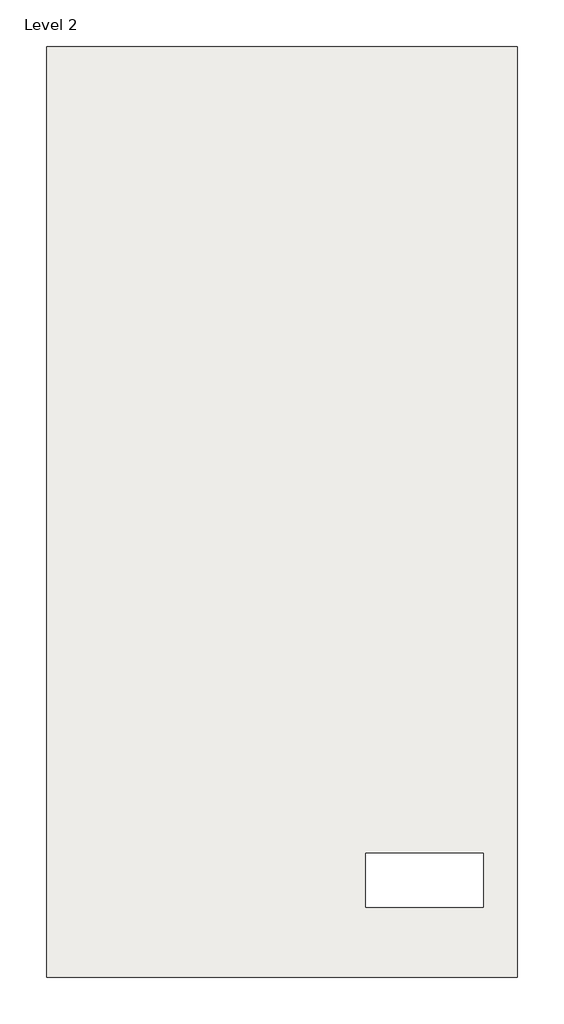
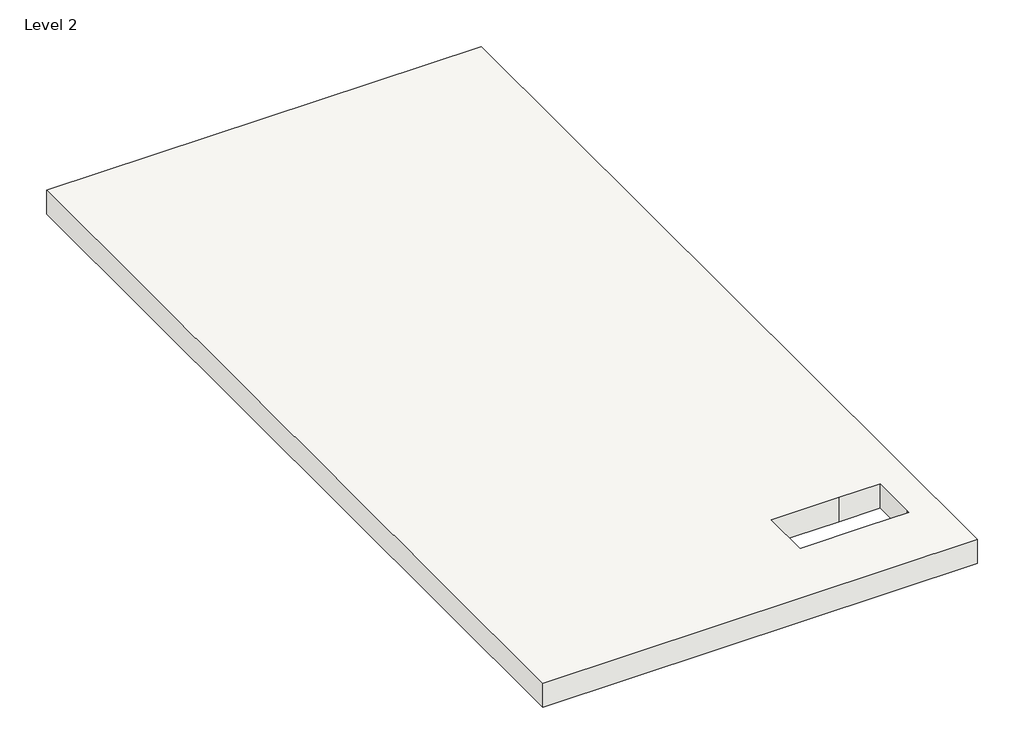
# One storey: 1 roof.
"""IFC4 building model written with IfcOpenShell, lengths in millimetres."""

from ifc_helpers import new_model, si_unit, frame, origin, place, context, project, spatial, polyline, outline, extrude, element, save

model = new_model("IFC4")

# Units and contexts
model_context = context("Model", 3, world=origin())
ifc_project = project(units=[si_unit("LENGTHUNIT", "METRE", prefix="MILLI")], contexts=[model_context])

# Site, building, storey
site = spatial("IfcSite", under=ifc_project)
building = spatial("IfcBuilding", under=site)
storey = spatial("IfcBuildingStorey", under=building, Name="Level 2", Elevation=3048.0)

# Roof
placement = place(None, origin())
element("IfcRoof", 1, ObjectType="Steel Truss - Insulation on Metal Deck - EPDM", at=placement, inside=storey, context=model_context, shape_type="SweptSolid", body=[
    extrude(outline(polyline([(-7777.408395, 15474.0151182), (1569.791605, 15474.0151182), (1569.791605, -3017.1848818), (-7777.408395, -3017.1848818), (-7777.408395, 15474.0151182)]), holes=[polyline([(-1440.108395, -604.1848818), (-1440.108395, -1620.1848818), (7.691605, -1620.1848818), (896.691605, -1620.1848818), (896.691605, -1601.1348818), (896.691605, -1543.9848818), (896.691605, -553.3848818), (7.691605, -553.3848818), (-1440.108395, -553.3848818), (-1440.108395, -604.1848818)])]), frame((0.0, 0.0, 3048.0), z_axis=(0.0, 0.0, 1.0), x_axis=(1.0, 0.0, 0.0)), (0.0, 0.0, 1.0), 546.1),
])

save(model, "model.ifc")

# Revit data of these elements
# Type "Steel Truss - Insulation on Metal Deck - EPDM"
#   Assembly Code = "B1020"
#   Layers, outside or top first: 0' - 0 1/4" "Roofing, EPDM Membrane" (function 4); 0' - 5" "Rigid insulation" (function 3); 0' - 0 1/4" "Metal Deck" (function 1); 1' - 4" "Structure, Steel Bar Joist Layer" (function 1)
# Element 1 (IfcRoof, "Steel Truss - Insulation on Metal Deck - EPDM")
#   built-in parameter 1001705 = 11.7917 (stored number, unit not read)
#   built-in parameter 1001710 = 33615
#   Phase Created = New Construction
#   Materials on its faces: "Structure, Steel Bar Joist Layer", "Roofing, EPDM Membrane"
# Materials
#   "Roofing, EPDM Membrane": class "Generic", colour RGB 127 127 127, transparency 0, Description = "EPDM roof membrane", Cost = 0
#   "Rigid insulation": class "Generic", colour RGB 127 127 127, transparency 0, Description = "Rigid foam insulation board", Cost = 0
#   "Metal Deck": class "Metal", colour RGB 199 199 199, transparency 0, Description = "Steel, mill finish", Cost = 0
#   "Structure, Steel Bar Joist Layer": class "Metal", colour RGB 127 127 127, transparency 0, Description = "Bar joists, thermal airspace", Cost = 0
